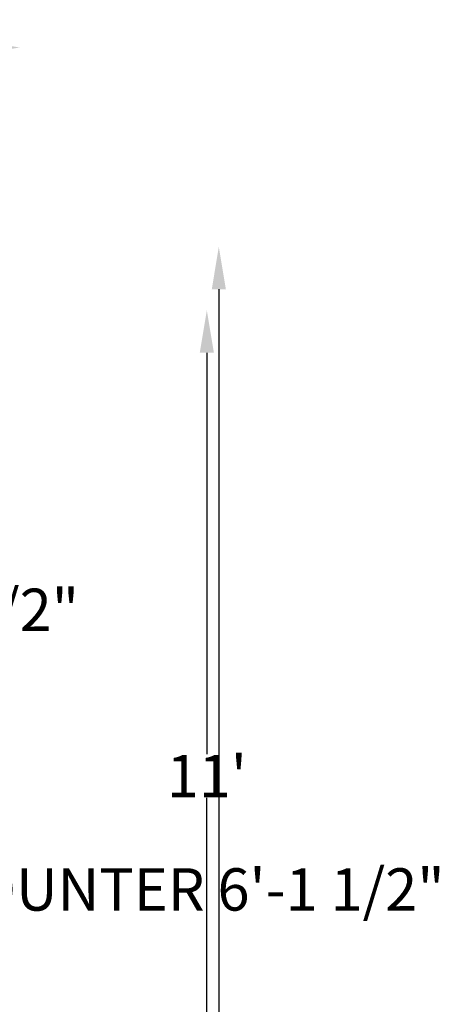
# Model space of a CAD drawing. Units: inches. Extents: x 2178 to 3409, y 1711 to 2279.
# Tile 8 of 8: x 2476 to 2536, y 2140 to 2279. Entities that reach past the tile are written whole.
import ezdxf

# ---------------------------------------------------------------- set-up
doc = ezdxf.new("R2010")
doc.units = ezdxf.units.IN
doc.layers.add('A-ANNO-DIMS', color=2, linetype='Continuous', lineweight=18)
doc.styles.get("Standard").update_dxf_attribs({"font": 'arial.ttf'})
doc.dimstyles.get("Standard").update_dxf_attribs({"dimtxt": 6, "dimasz": 6, "dimexe": 0.18, "dimexo": 0.0625, "dimgap": 0.09, "dimtad": 0, "dimtih": 1, "dimtoh": 1, "dimdec": 4, "dimzin": 0, "dimdsep": 46, "dimlunit": 4, "dimtxsty": 'Standard', "dimcen": 0.09, "dimse1": 1, "dimse2": 1, "dimadec": 0, "dimazin": 0, "dimtfac": 1, "dimtdec": 4, "dimtofl": 0, "dimtmove": 0, "dimatfit": 3, "dimfxl": 1, "dimtolj": 1, "dimtzin": 0, "dimarcsym": 0})

# ---------------------------------------------------------------- blocks, each defined once
blk = doc.blocks.new('*D21')
at = {"layer": 'A-ANNO-DIMS', "color": 0, "lineweight": -2, "transparency": 16777216}
for p, q in [((2502.61, 2232.04), (2502.61, 2175.14)), ((2502.61, 2112.04), (2502.61, 2168.94))]:
    blk.add_line(p, q, dxfattribs=at)
at = {"layer": 'A-ANNO-DIMS', "color": 0, "transparency": 16777216}
for points in [[(2501.61, 2232.04), (2503.61, 2232.04), (2502.61, 2238.04)], [(2501.61, 2112.04), (2503.61, 2112.04), (2502.61, 2106.04)]]:
    blk.add_solid(points, dxfattribs=at)
at = {"layer": 'Defpoints', "color": 0, "transparency": 16777216}
for p in [(2467.06, 2238.04), (2467.06, 2106.04), (2502.61, 2106.04)]:
    blk.add_point(p, dxfattribs=at)
at = {"layer": 'A-ANNO-DIMS', "color": 0, "transparency": 16777216, "insert": (2502.61, 2172.04), "char_height": 6, "attachment_point": 5}
blk.add_mtext("\\A1;11'", dxfattribs=at)
blk = doc.blocks.new('*D57')
at = {"layer": 'A-ANNO-DIMS', "color": 0, "lineweight": -2, "transparency": 16777216}
for p, q in [((2390.07, 2155.97), (2451.38, 2155.97)), ((2457.38, 2155.97), (2463.38, 2155.97))]:
    blk.add_line(p, q, dxfattribs=at)
at = {"layer": 'A-ANNO-DIMS', "color": 0, "transparency": 16777216}
for points in [[(2390.07, 2156.97), (2390.07, 2154.97), (2384.07, 2155.97)], [(2451.38, 2156.97), (2451.38, 2154.97), (2457.38, 2155.97)]]:
    blk.add_solid(points, dxfattribs=at)
at = {"layer": 'Defpoints', "color": 0, "transparency": 16777216}
for p in [(2384.07, 2166.96), (2457.38, 2166.96), (2457.38, 2155.97)]:
    blk.add_point(p, dxfattribs=at)
at = {"layer": 'A-ANNO-DIMS', "color": 0, "transparency": 16777216, "insert": (2500.29, 2155.97), "char_height": 6, "attachment_point": 5}
blk.add_mtext('\\A1;COUNTER 6\'-1 1/2"', dxfattribs=at)
blk = doc.blocks.new('*D58')
at = {"layer": 'A-ANNO-DIMS', "color": 0, "lineweight": -2, "transparency": 16777216}
for p, q in [((2468.38, 2218.23), (2468.38, 2198.79)), ((2468.38, 2172.96), (2468.38, 2192.4))]:
    blk.add_line(p, q, dxfattribs=at)
at = {"layer": 'A-ANNO-DIMS', "color": 0, "transparency": 16777216}
for points in [[(2467.38, 2218.23), (2469.38, 2218.23), (2468.38, 2224.23)], [(2467.38, 2172.96), (2469.38, 2172.96), (2468.38, 2166.96)]]:
    blk.add_solid(points, dxfattribs=at)
at = {"layer": 'Defpoints', "color": 0, "transparency": 16777216}
for p in [(2457.38, 2224.23), (2468.38, 2224.23), (2457.38, 2166.96)]:
    blk.add_point(p, dxfattribs=at)
at = {"layer": 'A-ANNO-DIMS', "color": 0, "transparency": 16777216, "insert": (2468.38, 2195.6), "char_height": 6, "attachment_point": 5}
blk.add_mtext('\\A1;4\'-9 1/2"', dxfattribs=at)
blk = doc.blocks.new('*D65')
at = {"layer": 'A-ANNO-DIMS', "color": 0, "lineweight": -2, "transparency": 16777216}
for p, q in [((2448.91, 2275.29), (2451.37, 2275.29)), ((2470.06, 2275.29), (2467.61, 2275.29))]:
    blk.add_line(p, q, dxfattribs=at)
at = {"layer": 'A-ANNO-DIMS', "color": 0, "transparency": 16777216}
for points in [[(2448.91, 2276.29), (2448.91, 2274.29), (2442.91, 2275.29)], [(2470.06, 2276.29), (2470.06, 2274.29), (2476.06, 2275.29)]]:
    blk.add_solid(points, dxfattribs=at)
at = {"layer": 'Defpoints', "color": 0, "transparency": 16777216}
for p in [(2476.06, 2275.29), (2442.91, 2247.04), (2476.06, 2247.04)]:
    blk.add_point(p, dxfattribs=at)
at = {"layer": 'A-ANNO-DIMS', "color": 0, "transparency": 16777216, "insert": (2459.49, 2275.29), "char_height": 6, "attachment_point": 5}
blk.add_mtext('\\A1;2\'-9"', dxfattribs=at)
blk = doc.blocks.new('*D75')
at = {"layer": 'A-ANNO-DIMS', "color": 0, "lineweight": -2, "transparency": 16777216}
for p, q in [((2504.31, 2241.04), (2504.31, 1998.2)), ((2504.31, 1749.04), (2504.31, 1991.89))]:
    blk.add_line(p, q, dxfattribs=at)
at = {"layer": 'A-ANNO-DIMS', "color": 0, "transparency": 16777216}
for points in [[(2503.31, 2241.04), (2505.31, 2241.04), (2504.31, 2247.04)], [(2503.31, 1749.04), (2505.31, 1749.04), (2504.31, 1743.04)]]:
    blk.add_solid(points, dxfattribs=at)
at = {"layer": 'Defpoints', "color": 0, "transparency": 16777216}
for p in [(2476.06, 2247.04), (2504.31, 2247.04), (2476.06, 1743.04)]:
    blk.add_point(p, dxfattribs=at)
at = {"layer": 'A-ANNO-DIMS', "color": 0, "transparency": 16777216, "insert": (2504.31, 1995.04), "char_height": 6, "attachment_point": 5}
blk.add_mtext('\\A1;42\'-0"', dxfattribs=at)

msp = doc.modelspace()

# ---------------------------------------------------------------- dimensions: what is measured, and where the dimension line sits
at = {"layer": 'A-ANNO-DIMS'}
dim = msp.add_linear_dim(base=(2476.06485, 2275.29256), p1=(2442.91353, 2247.04256), p2=(2476.06485, 2247.04256), dimstyle='Standard', override={"dimdec": 1, "dimlfac": 1, "dimrnd": 0, "dimzin": 1, "dimdsep": 46, "dimlunit": 4, "dimfrac": 2}, dxfattribs=at)
dim.commit()
dim.dimension.update_dxf_attribs({"geometry": '*D65', "text_midpoint": (2459.48919, 2275.29256)})
for base, p1, p2, override, picture, middle in [((2504.31485, 2247.04256), (2476.06485, 1743.04256), (2476.06485, 2247.04256), {"dimdec": 1, "dimlfac": 1, "dimrnd": 0, "dimzin": 1, "dimdsep": 46, "dimlunit": 4, "dimfrac": 2}, '*D75', (2504.31485, 1995.04256)), ((2502.61341, 2106.04256), (2467.06485, 2238.04256), (2467.06485, 2106.04256), {"dimclrd": 0, "dimclre": 0, "dimclrt": 0}, '*D21', (2502.61341, 2172.04256)), ((2468.3751, 2224.22693), (2457.37908, 2166.96329), (2457.37908, 2224.22693), {"dimdec": 1, "dimlfac": 1, "dimrnd": 0, "dimzin": 1, "dimdsep": 46, "dimlunit": 4, "dimfrac": 2}, '*D58', (2468.3751, 2195.59511))]:
    dim = msp.add_linear_dim(base=base, p1=p1, p2=p2, angle=90, dimstyle='Standard', override=override, dxfattribs=at)
    dim.commit()
    dim.dimension.update_dxf_attribs({"geometry": picture, "text_midpoint": middle})
dim = msp.add_linear_dim(base=(2457.37908, 2155.96728), p1=(2384.07233, 2166.96329), p2=(2457.37908, 2166.96329), text='COUNTER <>', dimstyle='Standard', override={"dimdec": 1, "dimlfac": 1, "dimrnd": 0, "dimzin": 1, "dimdsep": 46, "dimlunit": 4, "dimfrac": 2}, dxfattribs=at)
dim.commit()
dim.dimension.update_dxf_attribs({"geometry": '*D57', "text_midpoint": (2500.28559, 2155.96728)})

doc.saveas('drawing.dxf')
